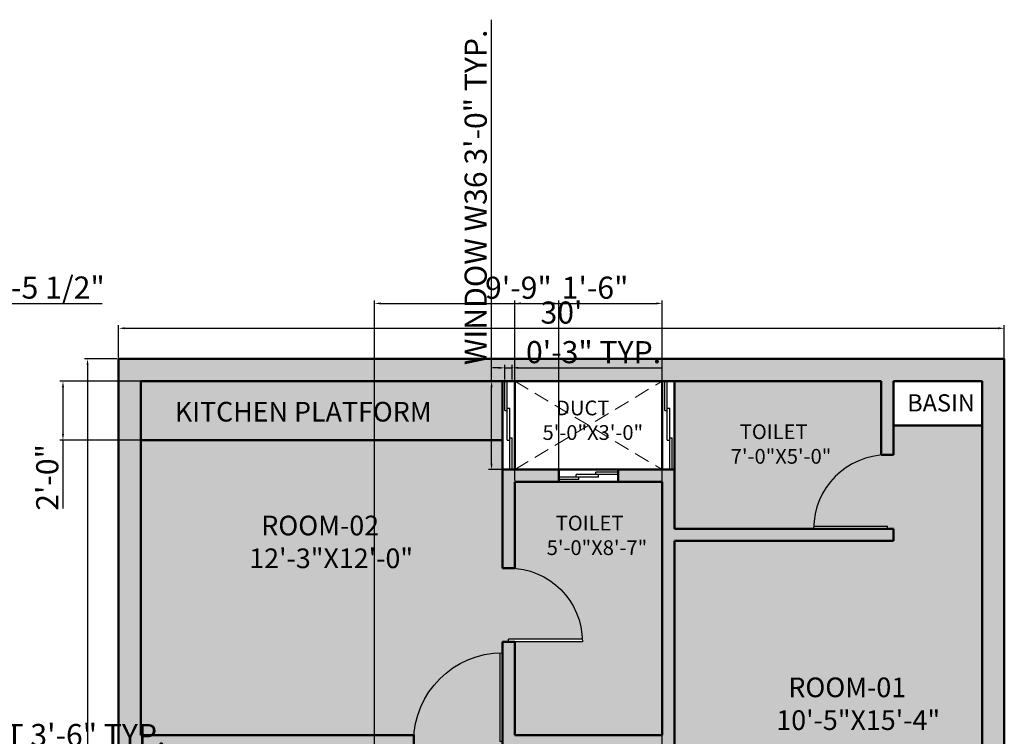
# Model space of a CAD drawing. Units: inches. Extents: x 3274 to 5176, y 1085 to 2172.
# Tile 10 of 16: x 3740 to 4140, y 1881 to 2172. Entities that reach past the tile are written whole.
import ezdxf

# ---------------------------------------------------------------- set-up
doc = ezdxf.new("R2010")
doc.units = ezdxf.units.IN
doc.linetypes.add('DASHED', pattern=[19.05, 12.7, -6.35])
for name, color, linetype, lineweight in [('A-ANNO-DIMS', 2, 'Continuous', 18), ('A-AREA-IDEN', 3, 'Continuous', 25), ('A-DOOR', 4, 'Continuous', 25), ('A-FLOR-OPEN', 7, 'DASHED', 18), ('A-FLOR-PATT', 252, 'Continuous', 13), ('A-GLAZ', 5, 'Continuous', 25), ('A-WALL', 7, 'Continuous', 50), ('A-WALL-PATT', 8, 'Continuous', 13)]:
    doc.layers.add(name, color=color, linetype=linetype, lineweight=lineweight)
doc.styles.get("Standard").update_dxf_attribs({"font": 'arial.ttf'})
doc.dimstyles.new('ISO-25', dxfattribs={"dimtxt": 9, "dimasz": 2.5, "dimexe": 1.25, "dimexo": 0.625, "dimtad": 1, "dimdec": 1, "dimlunit": 3, "dimtxsty": 'Standard', "dimcen": 2.5, "dimclrd": 4, "dimclre": 4, "dimclrt": 1, "dimadec": 0, "dimazin": 0, "dimtfac": 1, "dimtdec": 1, "dimtmove": 0, "dimatfit": 3, "dimfxl": 1, "dimarcsym": 0})

# ---------------------------------------------------------------- blocks, each defined once
blk = doc.blocks.new('*D65')
at = {"layer": 'A-ANNO-DIMS', "color": 0, "lineweight": -2, "transparency": 16777216}
for p, q in [((3779.73, 2035.11), (3779.73, 2048.22)), ((3782.23, 2046.97), (4137.23, 2046.97)), ((4139.73, 2035.11), (4139.73, 2048.22))]:
    blk.add_line(p, q, dxfattribs=at)
at = {"layer": 'A-ANNO-DIMS', "color": 0, "transparency": 16777216}
for points in [[(3782.23, 2047.39), (3782.23, 2046.56), (3779.73, 2046.97)], [(4137.23, 2047.39), (4137.23, 2046.56), (4139.73, 2046.97)]]:
    blk.add_solid(points, dxfattribs=at)
at = {"layer": 'Defpoints', "color": 0, "transparency": 16777216}
for p in [(4139.73, 2046.97), (3779.73, 2034.48), (4139.73, 2034.48)]:
    blk.add_point(p, dxfattribs=at)
at = {"layer": 'A-ANNO-DIMS', "color": 0, "transparency": 16777216, "insert": (3959.73, 2052.2), "char_height": 9, "attachment_point": 5}
blk.add_mtext("30'", dxfattribs=at)
blk = doc.blocks.new('*D66')
at = {"layer": 'A-ANNO-DIMS', "color": 0, "lineweight": -2, "transparency": 16777216}
for p, q in [((3779.1, 2034.48), (3765.87, 2034.48)), ((3767.12, 2031.98), (3767.12, 1676.98)), ((3779.1, 1674.48), (3765.87, 1674.48))]:
    blk.add_line(p, q, dxfattribs=at)
at = {"layer": 'A-ANNO-DIMS', "color": 0, "transparency": 16777216}
for points in [[(3766.71, 2031.98), (3767.54, 2031.98), (3767.12, 2034.48)], [(3766.71, 1676.98), (3767.54, 1676.98), (3767.12, 1674.48)]]:
    blk.add_solid(points, dxfattribs=at)
at = {"layer": 'Defpoints', "color": 0, "transparency": 16777216}
for p in [(3779.73, 2034.48), (3767.12, 1674.48), (3779.73, 1674.48)]:
    blk.add_point(p, dxfattribs=at)
at = {"layer": 'A-ANNO-DIMS', "color": 0, "transparency": 16777216, "insert": (3761.9, 1854.48), "char_height": 9, "attachment_point": 5, "rotation": 90}
blk.add_mtext("30'", dxfattribs=at)
blk = doc.blocks.new('1')
for p, q in [((0, 36), (0, 0)), ((1, 36), (1, 0)), ((0, 0), (1, 0))]:
    blk.add_line(p, q)
blk.add_arc((0, 0), 36, 0, 90)
blk = doc.blocks.new('2')
for p, q in [((0, 30), (0, 0)), ((1, 30), (1, 0)), ((0, 0), (1, 0))]:
    blk.add_line(p, q)
blk.add_arc((0, 0), 30, 0, 90)
blk = doc.blocks.new('WIN-24')
for p, q in [((4552.19, 1485.35), (4536.19, 1485.35)), ((4560.19, 1486.35), (4543.19, 1486.35)), ((4543.19, 1485.35), (4543.19, 1486.35)), ((4544.19, 1484.35), (4544.19, 1485.35)), ((4551.19, 1486.35), (4551.19, 1487.35)), ((4560.19, 1487.35), (4551.19, 1487.35)), ((4552.19, 1485.35), (4552.19, 1486.35)), ((4544.19, 1484.35), (4536.19, 1484.35))]:
    blk.add_line(p, q)
blk = doc.blocks.new('WIN-36')
for p, q in [((4514.19, 1512.35), (4514.19, 1524.35)), ((4515.19, 1500.35), (4515.19, 1524.35)), ((4515.19, 1513.35), (4516.19, 1513.35)), ((4516.19, 1488.35), (4516.19, 1513.35)), ((4514.19, 1512.35), (4515.19, 1512.35)), ((4516.19, 1501.35), (4517.19, 1501.35)), ((4517.19, 1488.35), (4517.19, 1501.35)), ((4515.19, 1500.35), (4516.19, 1500.35))]:
    blk.add_line(p, q)
blk = doc.blocks.new('*D122')
at = {"layer": 'A-ANNO-DIMS', "color": 4, "lineweight": -2, "transparency": 16777216}
for p, q in [((3931.33, 2025.48), (3931.33, 2172.47)), ((3936.1, 2025.48), (3930.08, 2025.48)), ((3931.33, 1991.98), (3931.33, 2022.98)), ((3936.1, 1989.48), (3930.08, 1989.48))]:
    blk.add_line(p, q, dxfattribs=at)
at = {"layer": 'A-ANNO-DIMS', "color": 4, "transparency": 16777216}
for points in [[(3930.91, 2022.98), (3931.75, 2022.98), (3931.33, 2025.48)], [(3930.91, 1991.98), (3931.75, 1991.98), (3931.33, 1989.48)]]:
    blk.add_solid(points, dxfattribs=at)
at = {"layer": 'Defpoints', "color": 0, "transparency": 16777216}
for p in [(3931.33, 2025.48), (3936.73, 2025.48), (3936.73, 1989.48)]:
    blk.add_point(p, dxfattribs=at)
at = {"layer": 'A-ANNO-DIMS', "color": 1, "transparency": 16777216, "insert": (3926.04, 2100.22), "char_height": 9, "attachment_point": 5, "rotation": 90}
blk.add_mtext('WINDOW W36 3\'-0" TYP.', dxfattribs=at)
blk = doc.blocks.new('*D123')
at = {"layer": 'A-ANNO-DIMS', "color": 4, "lineweight": -2, "transparency": 16777216}
for p, q in [((3934.23, 2030.88), (3931.73, 2030.88)), ((3936.73, 2026.11), (3936.73, 2032.13)), ((3936.73, 2030.88), (3939.73, 2030.88)), ((3939.73, 2026.11), (3939.73, 2032.13)), ((3942.23, 2030.88), (4000.84, 2030.88))]:
    blk.add_line(p, q, dxfattribs=at)
at = {"layer": 'A-ANNO-DIMS', "color": 4, "transparency": 16777216}
for points in [[(3934.23, 2031.3), (3934.23, 2030.47), (3936.73, 2030.88)], [(3942.23, 2031.3), (3942.23, 2030.47), (3939.73, 2030.88)]]:
    blk.add_solid(points, dxfattribs=at)
at = {"layer": 'Defpoints', "color": 0, "transparency": 16777216}
for p in [(3939.73, 2030.88), (3936.73, 2025.48), (3939.73, 2025.48)]:
    blk.add_point(p, dxfattribs=at)
at = {"layer": 'A-ANNO-DIMS', "color": 1, "transparency": 16777216, "insert": (3972.78, 2036.11), "char_height": 9, "attachment_point": 5}
blk.add_mtext('0\'-3" TYP.', dxfattribs=at)
blk = doc.blocks.new('*D130')
at = {"layer": 'A-ANNO-DIMS', "color": 4, "lineweight": -2, "transparency": 16777216}
for p, q in [((3648.04, 1880.86), (3648.04, 1873.91)), ((3690.17, 1880.86), (3690.17, 1873.91)), ((3650.54, 1875.16), (3687.67, 1875.16)), ((3690.17, 1875.16), (3801.39, 1875.16))]:
    blk.add_line(p, q, dxfattribs=at)
at = {"layer": 'A-ANNO-DIMS', "color": 4, "transparency": 16777216}
for points in [[(3650.54, 1875.58), (3650.54, 1874.75), (3648.04, 1875.16)], [(3687.67, 1875.58), (3687.67, 1874.75), (3690.17, 1875.16)]]:
    blk.add_solid(points, dxfattribs=at)
at = {"layer": 'Defpoints', "color": 0, "transparency": 16777216}
for p in [(3648.04, 1881.48), (3690.17, 1881.48), (3690.17, 1875.16)]:
    blk.add_point(p, dxfattribs=at)
at = {"layer": 'A-ANNO-DIMS', "color": 1, "transparency": 16777216, "insert": (3747.03, 1880.39), "char_height": 9, "attachment_point": 5}
blk.add_mtext('TV UNIT 3\'-6" TYP.', dxfattribs=at)
blk = doc.blocks.new('*D177')
at = {"layer": 'A-ANNO-DIMS', "color": 4, "lineweight": -2, "transparency": 16777216}
for p, q in [((3694.98, 1945.45), (3694.98, 2058.33)), ((3697.48, 2057.08), (3721.8, 2057.08)), ((3724.3, 1882.11), (3724.3, 2058.33)), ((3724.3, 2057.08), (3773.1, 2057.08))]:
    blk.add_line(p, q, dxfattribs=at)
at = {"layer": 'A-ANNO-DIMS', "color": 4, "transparency": 16777216}
for points in [[(3697.48, 2057.5), (3697.48, 2056.67), (3694.98, 2057.08)], [(3721.8, 2057.5), (3721.8, 2056.67), (3724.3, 2057.08)]]:
    blk.add_solid(points, dxfattribs=at)
at = {"layer": 'Defpoints', "color": 0, "transparency": 16777216}
for p in [(3724.3, 2057.08), (3694.98, 1944.83), (3724.3, 1881.48)]:
    blk.add_point(p, dxfattribs=at)
at = {"layer": 'A-ANNO-DIMS', "color": 1, "transparency": 16777216, "insert": (3749.95, 2062.36), "char_height": 9, "attachment_point": 5}
blk.add_mtext('2\'-5 1/2"', dxfattribs=at)
blk = doc.blocks.new('*D208')
at = {"layer": 'A-ANNO-DIMS', "color": 4, "lineweight": -2, "transparency": 16777216}
for p, q in [((3935.1, 2025.48), (3755.88, 2025.48)), ((3757.13, 2022.98), (3757.13, 2003.98)), ((3935.1, 2001.48), (3755.88, 2001.48)), ((3757.13, 2001.48), (3757.13, 1973.66))]:
    blk.add_line(p, q, dxfattribs=at)
at = {"layer": 'A-ANNO-DIMS', "color": 4, "transparency": 16777216}
for points in [[(3756.71, 2022.98), (3757.55, 2022.98), (3757.13, 2025.48)], [(3756.71, 2003.98), (3757.55, 2003.98), (3757.13, 2001.48)]]:
    blk.add_solid(points, dxfattribs=at)
at = {"layer": 'Defpoints', "color": 0, "transparency": 16777216}
for p in [(3935.73, 2025.48), (3757.13, 2001.48), (3935.73, 2001.48)]:
    blk.add_point(p, dxfattribs=at)
at = {"layer": 'A-ANNO-DIMS', "color": 1, "transparency": 16777216, "insert": (3751.91, 1986.32), "char_height": 9, "attachment_point": 5, "rotation": 90}
blk.add_mtext('2\'-0"', dxfattribs=at)
blk = doc.blocks.new('*D212')
at = {"layer": 'A-ANNO-DIMS', "color": 4, "lineweight": -2, "transparency": 16777216}
for p, q in [((3883.73, 1877.11), (3883.73, 2058.33)), ((3886.23, 2057.08), (3998.23, 2057.08)), ((4000.73, 1841.11), (4000.73, 2058.33))]:
    blk.add_line(p, q, dxfattribs=at)
at = {"layer": 'A-ANNO-DIMS', "color": 4, "transparency": 16777216}
for points in [[(3886.23, 2057.5), (3886.23, 2056.67), (3883.73, 2057.08)], [(3998.23, 2057.5), (3998.23, 2056.67), (4000.73, 2057.08)]]:
    blk.add_solid(points, dxfattribs=at)
at = {"layer": 'Defpoints', "color": 0, "transparency": 16777216}
for p in [(4000.73, 2057.08), (3883.73, 1876.48), (4000.73, 1840.48)]:
    blk.add_point(p, dxfattribs=at)
at = {"layer": 'A-ANNO-DIMS', "color": 1, "transparency": 16777216, "insert": (3942.23, 2062.3), "char_height": 9, "attachment_point": 5}
blk.add_mtext('9\'-9"', dxfattribs=at)
blk = doc.blocks.new('*D215')
at = {"layer": 'A-ANNO-DIMS', "color": 4, "lineweight": -2, "transparency": 16777216}
for p, q in [((3940.73, 1985.11), (3940.73, 2058.33)), ((3943.23, 2057.08), (3956.23, 2057.08)), ((3958.73, 1985.11), (3958.73, 2058.33)), ((3958.73, 2057.08), (3985.56, 2057.08))]:
    blk.add_line(p, q, dxfattribs=at)
at = {"layer": 'A-ANNO-DIMS', "color": 4, "transparency": 16777216}
for points in [[(3943.23, 2057.5), (3943.23, 2056.67), (3940.73, 2057.08)], [(3956.23, 2057.5), (3956.23, 2056.67), (3958.73, 2057.08)]]:
    blk.add_solid(points, dxfattribs=at)
at = {"layer": 'Defpoints', "color": 0, "transparency": 16777216}
for p in [(3958.73, 2057.08), (3940.73, 1984.48), (3958.73, 1984.48)]:
    blk.add_point(p, dxfattribs=at)
at = {"layer": 'A-ANNO-DIMS', "color": 1, "transparency": 16777216, "insert": (3973.39, 2062.3), "char_height": 9, "attachment_point": 5}
blk.add_mtext('1\'-6"', dxfattribs=at)

msp = doc.modelspace()

# ---------------------------------------------------------------- hatches: boundary and pattern name
at = {"layer": 'A-FLOR-PATT'}
h = msp.add_hatch(color=256, dxfattribs=at)
h.dxf.hatch_style = 1
h.paths.add_polyline_path([(3935.73, 2001.48), (3935.73, 2025.48), (3788.73, 2025.48), (3788.73, 2001.48)])
h.paths.add_polyline_path([(3799.76, 2004.54), (3916.77, 2004.54), (3916.77, 2021.03), (3799.76, 2021.03)], flags=24)
h = msp.add_hatch(color=256, dxfattribs=at)
h.dxf.hatch_style = 1
h.paths.add_polyline_path([(4130.73, 2007.48), (4094.73, 2007.48), (4094.73, 1995.48), (4092.23, 1995.48, 0.404482), (4062.25, 1966.48), (4092.23, 1966.48), (4092.23, 1965.48), (4094.73, 1965.48), (4094.73, 1960.48), (4005.73, 1960.48), (4005.73, 1876.48), (4039.23, 1876.48, -0.394001), (4005.73, 1840.57), (4005.73, 1800.48), (4130.73, 1800.48)])
h.paths.add_polyline_path([(4089.73, 1995.38), (4089.73, 2025.48), (4005.73, 2025.48), (4005.73, 1965.48), (4062.23, 1965.48, -0.389983)])
h.paths.add_polyline_path([(4039.22, 1875.48), (4003.23, 1875.48), (4003.23, 1876.48), (4000.73, 1876.48), (4000.73, 1840.48), (4003.23, 1840.48, 0.4061)])
h.paths.add_polyline_path([(4043.84, 1879.07), (4112.24, 1879.07), (4112.24, 1908.93), (4043.84, 1908.93)], flags=24)
h.paths.add_polyline_path([(4026.66, 1988.49), (4068.63, 1988.49), (4068.63, 2010.88), (4026.66, 2010.88)], flags=24)
h = msp.add_hatch(color=256, dxfattribs=at)
h.dxf.hatch_style = 1
h.paths.add_polyline_path([(3938.23, 1949.48), (3935.73, 1949.48), (3935.73, 2001.48), (3788.73, 2001.48), (3788.73, 1881.48), (3899.82, 1881.48, -0.394001), (3935.73, 1914.98), (3935.73, 1919.48), (3938.23, 1919.48), (3938.23, 1920.48), (3968.21, 1920.48, 0.404482)])
h.paths.add_polyline_path([(3934.73, 1914.97, 0.4061), (3899.73, 1878.98), (3899.73, 1876.48), (3935.73, 1876.48), (3935.73, 1878.98), (3934.73, 1878.98)])
h.paths.add_polyline_path([(4000.73, 1984.48), (3940.73, 1984.48), (3940.73, 1949.38, -0.389983), (3968.23, 1919.48), (3940.73, 1919.48), (3940.73, 1881.48), (4000.73, 1881.48)])
h.paths.add_polyline_path([(3829.62, 1944.89), (3898.01, 1944.89), (3898.01, 1974.74), (3829.62, 1974.74)], flags=24)
h.paths.add_polyline_path([(3951.89, 1951.36), (3993.86, 1951.36), (3993.86, 1973.74), (3951.89, 1973.74)], flags=24)
at = {"layer": 'A-WALL-PATT'}
h = msp.add_hatch(color=256, dxfattribs=at)
h.dxf.hatch_style = 1
h.paths.add_polyline_path([(3848.73, 1820.48), (3823.73, 1820.48), (3823.73, 1840.48), (3818.73, 1840.48), (3818.73, 1815.48), (3848.73, 1815.48)], flags=17)
h.paths.add_polyline_path([(3788.73, 1876.48), (3878.73, 1876.48), (3878.73, 1815.48), (3899.73, 1815.48), (3899.73, 1820.48), (3883.73, 1820.48), (3883.73, 1876.48), (3899.73, 1876.48), (3899.73, 1881.48), (3788.73, 1881.48), (3788.73, 2025.48), (4089.73, 2025.48), (4089.73, 1995.48), (4094.73, 1995.48), (4094.73, 2025.48), (4130.73, 2025.48), (4130.73, 1776.48), (4098.23, 1776.48), (4098.23, 1767.48), (4130.73, 1767.48), (4130.73, 1683.48), (4088.73, 1683.48), (4088.73, 1674.48), (4139.73, 1674.48), (4139.73, 2034.48), (3779.73, 2034.48), (3779.73, 1674.48), (3812.73, 1674.48), (3812.73, 1683.48), (3788.73, 1683.48)])
h.paths.add_polyline_path([(4005.73, 1989.48), (3982.73, 1989.48), (3982.73, 1984.48), (4000.73, 1984.48), (4000.73, 1881.48), (3940.73, 1881.48), (3940.73, 1919.48), (3938.23, 1919.48), (3935.73, 1919.48), (3935.73, 1876.48), (4005.73, 1876.48), (4005.73, 1960.48), (4094.73, 1960.48), (4094.73, 1965.48), (4005.73, 1965.48)], flags=17)
h.paths.add_polyline_path([(3958.73, 1989.48), (3935.73, 1989.48), (3935.73, 1949.48), (3940.73, 1949.48), (3940.73, 1984.48), (3958.73, 1984.48)], flags=17)
h.paths.add_polyline_path([(4038.23, 1776.48), (4005.73, 1776.48), (4005.73, 1840.48), (4000.73, 1840.48), (4000.73, 1776.48), (3993.73, 1776.48), (3993.73, 1771.98), (3993.73, 1767.48), (4038.23, 1767.48)], flags=17)
h.paths.add_polyline_path([(3940.73, 1767.48), (3945.73, 1767.48), (3945.73, 1776.48), (3940.73, 1776.48), (3940.73, 1820.48), (3935.73, 1820.48), (3935.73, 1683.48), (3884.73, 1683.48), (3884.73, 1674.48), (3940.73, 1674.48)], flags=17)
h.paths.add_polyline_path([(4016.73, 1683.48), (4000.73, 1683.48), (4000.73, 1674.48), (4016.73, 1674.48)], flags=17)

# ---------------------------------------------------------------- linework, layer by layer
at = {"layer": 'A-FLOR-OPEN', "ltscale": 0.5}
for p, q in [((3940.73, 2025.48), (4000.73, 1989.48)), ((3940.73, 1989.48), (4000.73, 2025.48))]:
    msp.add_line(p, q, dxfattribs=at)
at = {"layer": 'A-WALL'}
for p, q in [((3788.73, 2025.48), (4089.73, 2025.48)), ((3788.73, 1881.48), (3788.73, 2025.48)), ((3935.73, 1949.48), (3935.73, 2025.48)), ((3940.73, 1989.48), (3940.73, 2025.48)), ((4000.73, 2025.48), (4000.73, 1989.48)), ((4005.73, 2025.48), (4005.73, 1965.48)), ((4089.73, 2025.48), (4089.73, 1995.48)), ((4094.73, 2025.48), (4130.73, 2025.48)), ((4094.73, 2025.48), (4094.73, 1995.48)), ((4130.73, 2025.48), (4130.73, 1776.48)), ((4094.73, 2007.48), (4130.73, 2007.48)), ((3788.73, 2001.48), (3935.73, 2001.48)), ((4089.73, 1995.48), (4094.73, 1995.48)), ((3935.73, 1989.48), (4005.73, 1989.48)), ((3958.73, 1984.48), (3958.73, 1989.48)), ((3982.73, 1984.48), (3982.73, 1989.48)), ((3940.73, 1984.48), (4000.73, 1984.48)), ((3940.73, 1949.48), (3940.73, 1984.48)), ((4000.73, 1984.48), (4000.73, 1881.48)), ((4005.73, 1965.48), (4094.73, 1965.48)), ((4094.73, 1965.48), (4094.73, 1960.48)), ((4005.73, 1960.48), (4094.73, 1960.48)), ((4005.73, 1960.48), (4005.73, 1876.48)), ((3935.73, 1949.48), (3940.73, 1949.48)), ((3935.73, 1919.48), (3940.73, 1919.48)), ((3935.73, 1876.48), (3935.73, 1919.48)), ((3940.73, 1881.48), (3940.73, 1919.48)), ((3788.73, 1881.48), (3899.73, 1881.48)), ((3899.73, 1876.48), (3899.73, 1881.48)), ((3940.73, 1881.48), (4000.73, 1881.48))]:
    msp.add_line(p, q, dxfattribs=at)
msp.add_lwpolyline([(3940.73, 1674.48), (3779.73, 1674.48), (3779.73, 2034.48), (4139.73, 2034.48), (4139.73, 1674.48), (3940.73, 1674.48)], dxfattribs=at)

# ---------------------------------------------------------------- block references
at = {"layer": 'A-DOOR', "rotation": 89.99999999999999}
msp.add_blockref('2', (4092.23, 1965.48), dxfattribs=at)
at = {"layer": 'A-DOOR', "xscale": -1, "rotation": 270}
msp.add_blockref('2', (3938.23, 1919.48), dxfattribs=at)
at = {"layer": 'A-DOOR', "xscale": -1}
msp.add_blockref('1', (3935.73, 1878.98), dxfattribs=at)
at = {"layer": 'A-GLAZ'}
for name, p in [('WIN-36', (-577.46, 501.13)), ('WIN-36', (-512.46, 501.13)), ('WIN-24', (-577.46, 501.13))]:
    msp.add_blockref(name, p, dxfattribs=at)

# ---------------------------------------------------------------- texts
at = {"layer": 'A-AREA-IDEN', "attachment_point": 1}
for s, width, heights, insert, char_height in [('KITCHEN PLATFORM', 147.1149, [0], (3802.58, 2017.05), 8), ('   DUCT\\P5\'-0"X3\'-0"', 58.0121, [16.24], (3952.06, 2017.57), 6), ('BASIN', 147.1149, [0], (4100.28, 2020.14), 7), ('  TOILET\\P7\'-0"X5\'-0"', 58.0121, [16.24], (4028.55, 2007.9), 6), ('  ROOM-02\\P12\'-3"X12\'-0"', 58.0121, [0], (3832.84, 1970.76), 8), ('  TOILET\\P5\'-0"X8\'-7"', 58.0121, [16.24], (3953.74, 1970.76), 6), ('  ROOM-01\\P10\'-5"X15\'-4"', 58.0121, [0], (4047.06, 1904.95), 8)]:
    msp.add_mtext_dynamic_manual_height_columns(s, width=width, gutter_width=30, heights=heights, dxfattribs=dict(at, insert=insert, char_height=char_height))

# ---------------------------------------------------------------- dimensions: what is measured, and where the dimension line sits
at = {"layer": 'A-ANNO-DIMS'}
dim = msp.add_linear_dim(base=(3931.33, 2025.48), p1=(3936.73, 1989.48), p2=(3936.73, 2025.48), angle=90, text='WINDOW W36 <> TYP.', dimstyle='ISO-25', override={"dimdec": 1, "dimrnd": 0, "dimzin": 1, "dimlunit": 4, "dimfrac": 2}, dxfattribs=at)
dim.commit()
dim.dimension.update_dxf_attribs({"geometry": '*D122', "text_midpoint": (3926.04, 2100.22)})
for base, p1, p2, override, picture, middle in [((3724.3, 2057.08), (3694.98, 1944.83), (3724.3, 1881.48), {"dimdec": 1, "dimlfac": 1, "dimrnd": 0, "dimzin": 1, "dimdsep": 46, "dimlunit": 4, "dimfrac": 2}, '*D177', (3749.95, 2062.36)), ((4000.73, 2057.08), (3883.73, 1876.48), (4000.73, 1840.48), {"dimdec": 1, "dimlfac": 1, "dimrnd": 0, "dimzin": 1, "dimdsep": 46, "dimlunit": 4, "dimfrac": 2}, '*D212', (3942.23, 2062.3)), ((3958.73, 2057.08), (3940.73, 1984.48), (3958.73, 1984.48), {"dimdec": 1, "dimlfac": 1, "dimrnd": 0, "dimzin": 1, "dimdsep": 46, "dimlunit": 4, "dimfrac": 2}, '*D215', (3973.39, 2062.3)), ((4139.73, 2046.97), (3779.73, 2034.48), (4139.73, 2034.48), {"dimclrd": 0, "dimclre": 0, "dimclrt": 0}, '*D65', (3959.73, 2052.2))]:
    dim = msp.add_linear_dim(base=base, p1=p1, p2=p2, dimstyle='ISO-25', override=override, dxfattribs=at)
    dim.commit()
    dim.dimension.update_dxf_attribs({"geometry": picture, "text_midpoint": middle})
for base, p1, p2, text, picture, middle in [((3939.73, 2030.88), (3936.73, 2025.48), (3939.73, 2025.48), '<> TYP.', '*D123', (3972.78, 2036.11)), ((3690.17, 1875.16), (3648.04, 1881.48), (3690.17, 1881.48), 'TV UNIT <> TYP.', '*D130', (3747.03, 1880.39))]:
    dim = msp.add_linear_dim(base=base, p1=p1, p2=p2, text=text, dimstyle='ISO-25', override={"dimdec": 1, "dimrnd": 0, "dimzin": 1, "dimlunit": 4, "dimfrac": 2}, dxfattribs=at)
    dim.commit()
    dim.dimension.update_dxf_attribs({"geometry": picture, "text_midpoint": middle})
for base, p1, p2, override, picture, middle in [((3767.12, 1674.48), (3779.73, 2034.48), (3779.73, 1674.48), {"dimclrd": 0, "dimclre": 0, "dimclrt": 0}, '*D66', (3761.9, 1854.48)), ((3757.13, 2001.48), (3935.73, 2025.48), (3935.73, 2001.48), {"dimdec": 1, "dimlfac": 1, "dimrnd": 0, "dimzin": 1, "dimdsep": 46, "dimlunit": 4, "dimfrac": 2}, '*D208', (3751.91, 1986.32))]:
    dim = msp.add_linear_dim(base=base, p1=p1, p2=p2, angle=90, dimstyle='ISO-25', override=override, dxfattribs=at)
    dim.commit()
    dim.dimension.update_dxf_attribs({"geometry": picture, "text_midpoint": middle})

doc.saveas('drawing.dxf')
